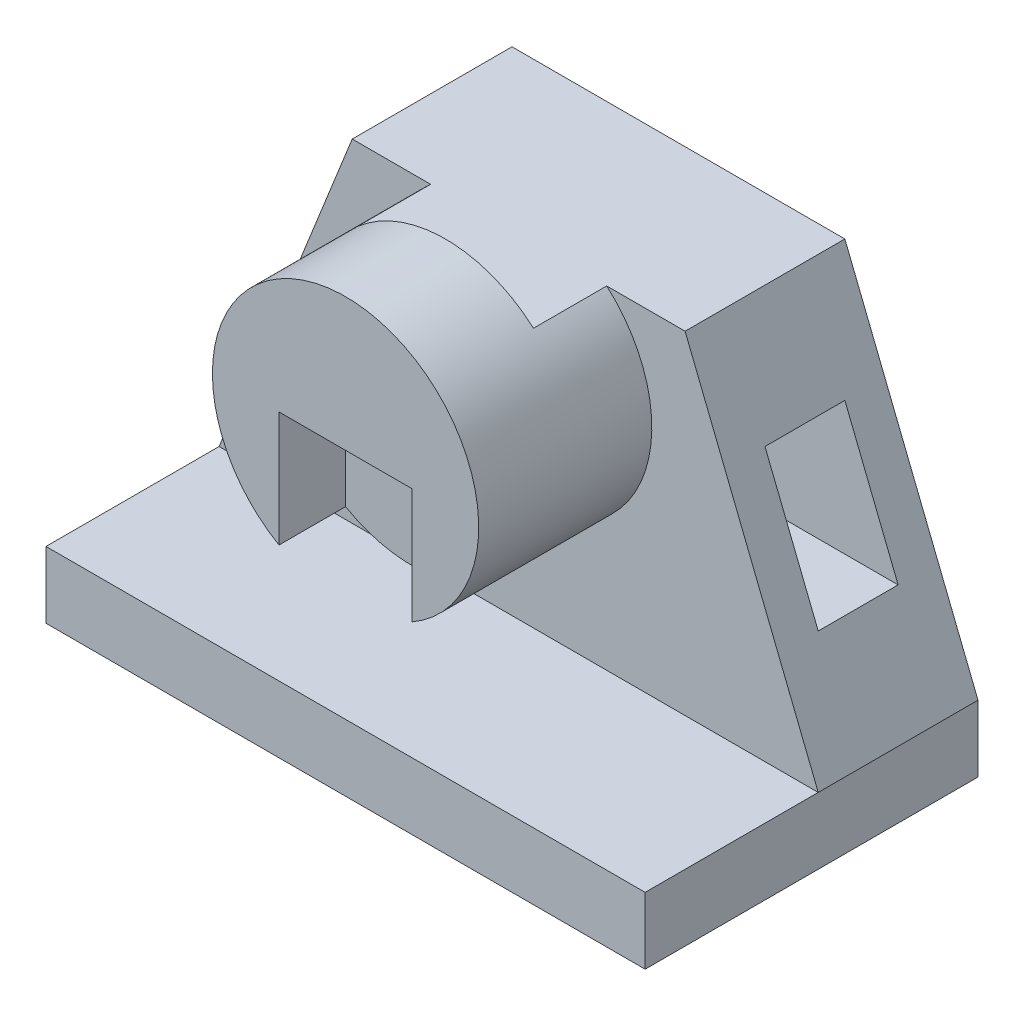
ISO-10303-21;
HEADER;
FILE_DESCRIPTION(('STEP AP214'),'2;1');
FILE_NAME('part.step','',(''),(''),'','','');
FILE_SCHEMA(('AUTOMOTIVE_DESIGN { 1 0 10303 214 1 1 1 1 }'));
ENDSEC;
DATA;
#1=APPLICATION_CONTEXT('core data for automotive mechanical design processes');
#2=APPLICATION_PROTOCOL_DEFINITION('international standard','automotive_design',2000,#1);
#3=PRODUCT_CONTEXT('',#1,'mechanical');
#4=PRODUCT('Part','Part','',(#3));
#5=PRODUCT_RELATED_PRODUCT_CATEGORY('part','',(#4));
#6=PRODUCT_DEFINITION_FORMATION('','',#4);
#7=PRODUCT_DEFINITION_CONTEXT('part definition',#1,'design');
#8=PRODUCT_DEFINITION('design','',#6,#7);
#9=PRODUCT_DEFINITION_SHAPE('','',#8);
#10=(LENGTH_UNIT() NAMED_UNIT(*) SI_UNIT(.MILLI.,.METRE.));
#11=(NAMED_UNIT(*) PLANE_ANGLE_UNIT() SI_UNIT($,.RADIAN.));
#12=(NAMED_UNIT(*) SI_UNIT($,.STERADIAN.) SOLID_ANGLE_UNIT());
#13=UNCERTAINTY_MEASURE_WITH_UNIT(LENGTH_MEASURE(1.E-05),#10,'distance_accuracy_value','');
#14=(GEOMETRIC_REPRESENTATION_CONTEXT(3) GLOBAL_UNCERTAINTY_ASSIGNED_CONTEXT((#13)) GLOBAL_UNIT_ASSIGNED_CONTEXT((#10,
#11,#12)) REPRESENTATION_CONTEXT('',''));
#15=CARTESIAN_POINT('',(0.,0.,0.));
#16=DIRECTION('',(0.,0.,1.));
#17=DIRECTION('',(1.,0.,0.));
#18=AXIS2_PLACEMENT_3D('',#15,#16,#17);
#19=CARTESIAN_POINT('',(-3.44827586206896,1.37931034482759,24.));
#20=DIRECTION('',(-0.928476690885259,0.371390676354103,0.));
#21=DIRECTION('',(-0.371390676354104,-0.928476690885259,0.));
#22=AXIS2_PLACEMENT_3D('',#19,#20,#21);
#23=PLANE('',#22);
#24=DIRECTION('',(0.371390676354104,0.92847669088526,0.));
#25=VECTOR('',#24,1.);
#26=CARTESIAN_POINT('',(-3.44827586206896,1.37931034482759,18.));
#27=LINE('',#26,#25);
#28=CARTESIAN_POINT('',(5.99999999999999,25.,18.));
#29=VERTEX_POINT('',#28);
#30=CARTESIAN_POINT('',(14.,45.,18.));
#31=VERTEX_POINT('',#30);
#32=EDGE_CURVE('E167',#29,#31,#27,.T.);
#33=ORIENTED_EDGE('',*,*,#32,.F.);
#34=DIRECTION('',(0.,0.,1.));
#35=VECTOR('',#34,1.);
#36=CARTESIAN_POINT('',(5.99999999999999,25.,24.));
#37=LINE('',#36,#35);
#38=CARTESIAN_POINT('',(5.99999999999999,25.,6.00000000000001));
#39=VERTEX_POINT('',#38);
#40=EDGE_CURVE('E154',#39,#29,#37,.T.);
#41=ORIENTED_EDGE('',*,*,#40,.F.);
#42=DIRECTION('',(-0.371390676354104,-0.92847669088526,0.));
#43=VECTOR('',#42,1.);
#44=CARTESIAN_POINT('',(-3.44827586206896,1.37931034482759,6.));
#45=LINE('',#44,#43);
#46=CARTESIAN_POINT('',(14.,45.,6.00000000000001));
#47=VERTEX_POINT('',#46);
#48=EDGE_CURVE('E159',#47,#39,#45,.T.);
#49=ORIENTED_EDGE('',*,*,#48,.F.);
#50=DIRECTION('',(0.,0.,-1.));
#51=VECTOR('',#50,1.);
#52=CARTESIAN_POINT('',(14.,45.,24.));
#53=LINE('',#52,#51);
#54=EDGE_CURVE('E171',#31,#47,#53,.T.);
#55=ORIENTED_EDGE('',*,*,#54,.F.);
#56=EDGE_LOOP('',(#33,#41,#49,#55));
#57=FACE_BOUND('',#56,.T.);
#58=DIRECTION('',(0.371390676354104,0.928476690885259,0.));
#59=VECTOR('',#58,1.);
#60=CARTESIAN_POINT('',(-3.44827586206896,1.37931034482759,0.));
#61=LINE('',#60,#59);
#62=CARTESIAN_POINT('',(0.,10.,0.));
#63=VERTEX_POINT('',#62);
#64=CARTESIAN_POINT('',(20.,60.,0.));
#65=VERTEX_POINT('',#64);
#66=EDGE_CURVE('E242',#63,#65,#61,.T.);
#67=ORIENTED_EDGE('',*,*,#66,.F.);
#68=DIRECTION('',(0.,0.,-1.));
#69=VECTOR('',#68,1.);
#70=CARTESIAN_POINT('',(0.,10.,24.));
#71=LINE('',#70,#69);
#72=CARTESIAN_POINT('',(0.,10.,24.));
#73=VERTEX_POINT('',#72);
#74=EDGE_CURVE('E273',#73,#63,#71,.T.);
#75=ORIENTED_EDGE('',*,*,#74,.F.);
#76=DIRECTION('',(0.371390676354104,0.928476690885259,0.));
#77=VECTOR('',#76,1.);
#78=CARTESIAN_POINT('',(-3.44827586206896,1.37931034482759,24.));
#79=LINE('',#78,#77);
#80=CARTESIAN_POINT('',(20.,60.,24.));
#81=VERTEX_POINT('',#80);
#82=EDGE_CURVE('E247',#73,#81,#79,.T.);
#83=ORIENTED_EDGE('',*,*,#82,.T.);
#84=DIRECTION('',(0.,0.,-1.));
#85=VECTOR('',#84,1.);
#86=CARTESIAN_POINT('',(20.,60.,24.));
#87=LINE('',#86,#85);
#88=EDGE_CURVE('E257',#81,#65,#87,.T.);
#89=ORIENTED_EDGE('',*,*,#88,.T.);
#90=EDGE_LOOP('',(#67,#75,#83,#89));
#91=FACE_BOUND('',#90,.T.);
#92=ADVANCED_FACE('F41',(#57,#91),#23,.T.);
#93=CARTESIAN_POINT('',(81.0344827586207,32.4137931034483,24.));
#94=DIRECTION('',(0.928476690885259,0.371390676354104,0.));
#95=DIRECTION('',(-0.371390676354104,0.928476690885259,0.));
#96=AXIS2_PLACEMENT_3D('',#93,#94,#95);
#97=PLANE('',#96);
#98=DIRECTION('',(0.371390676354104,-0.928476690885259,0.));
#99=VECTOR('',#98,1.);
#100=CARTESIAN_POINT('',(81.0344827586207,32.4137931034483,18.));
#101=LINE('',#100,#99);
#102=CARTESIAN_POINT('',(76.,45.,18.));
#103=VERTEX_POINT('',#102);
#104=CARTESIAN_POINT('',(84.,25.,18.));
#105=VERTEX_POINT('',#104);
#106=EDGE_CURVE('E11',#103,#105,#101,.T.);
#107=ORIENTED_EDGE('',*,*,#106,.F.);
#108=DIRECTION('',(0.,0.,1.));
#109=VECTOR('',#108,1.);
#110=CARTESIAN_POINT('',(76.,45.,24.));
#111=LINE('',#110,#109);
#112=CARTESIAN_POINT('',(76.,45.,6.00000000000001));
#113=VERTEX_POINT('',#112);
#114=EDGE_CURVE('E48',#113,#103,#111,.T.);
#115=ORIENTED_EDGE('',*,*,#114,.F.);
#116=DIRECTION('',(-0.371390676354104,0.928476690885259,0.));
#117=VECTOR('',#116,1.);
#118=CARTESIAN_POINT('',(81.0344827586207,32.4137931034483,6.00000000000001));
#119=LINE('',#118,#117);
#120=CARTESIAN_POINT('',(84.,25.,6.));
#121=VERTEX_POINT('',#120);
#122=EDGE_CURVE('E283',#121,#113,#119,.T.);
#123=ORIENTED_EDGE('',*,*,#122,.F.);
#124=DIRECTION('',(0.,0.,-1.));
#125=VECTOR('',#124,1.);
#126=CARTESIAN_POINT('',(84.,25.,24.));
#127=LINE('',#126,#125);
#128=EDGE_CURVE('E276',#105,#121,#127,.T.);
#129=ORIENTED_EDGE('',*,*,#128,.F.);
#130=EDGE_LOOP('',(#107,#115,#123,#129));
#131=FACE_BOUND('',#130,.T.);
#132=DIRECTION('',(0.371390676354104,-0.928476690885259,0.));
#133=VECTOR('',#132,1.);
#134=CARTESIAN_POINT('',(81.0344827586207,32.4137931034483,0.));
#135=LINE('',#134,#133);
#136=CARTESIAN_POINT('',(70.,60.,0.));
#137=VERTEX_POINT('',#136);
#138=CARTESIAN_POINT('',(90.,10.,0.));
#139=VERTEX_POINT('',#138);
#140=EDGE_CURVE('E263',#137,#139,#135,.T.);
#141=ORIENTED_EDGE('',*,*,#140,.F.);
#142=DIRECTION('',(0.,0.,-1.));
#143=VECTOR('',#142,1.);
#144=CARTESIAN_POINT('',(70.,60.,24.));
#145=LINE('',#144,#143);
#146=CARTESIAN_POINT('',(70.,60.,24.));
#147=VERTEX_POINT('',#146);
#148=EDGE_CURVE('E267',#147,#137,#145,.T.);
#149=ORIENTED_EDGE('',*,*,#148,.F.);
#150=DIRECTION('',(0.371390676354104,-0.928476690885259,0.));
#151=VECTOR('',#150,1.);
#152=CARTESIAN_POINT('',(81.0344827586207,32.4137931034483,24.));
#153=LINE('',#152,#151);
#154=CARTESIAN_POINT('',(90.,10.,24.));
#155=VERTEX_POINT('',#154);
#156=EDGE_CURVE('E251',#147,#155,#153,.T.);
#157=ORIENTED_EDGE('',*,*,#156,.T.);
#158=DIRECTION('',(0.,0.,-1.));
#159=VECTOR('',#158,1.);
#160=CARTESIAN_POINT('',(90.,10.,24.));
#161=LINE('',#160,#159);
#162=EDGE_CURVE('E271',#155,#139,#161,.T.);
#163=ORIENTED_EDGE('',*,*,#162,.T.);
#164=EDGE_LOOP('',(#141,#149,#157,#163));
#165=FACE_BOUND('',#164,.T.);
#166=ADVANCED_FACE('F292',(#131,#165),#97,.T.);
#167=CARTESIAN_POINT('',(0.,60.,24.));
#168=DIRECTION('',(0.,1.,0.));
#169=DIRECTION('',(-1.,0.,0.));
#170=AXIS2_PLACEMENT_3D('',#167,#168,#169);
#171=PLANE('',#170);
#172=DIRECTION('',(1.,0.,0.));
#173=VECTOR('',#172,1.);
#174=CARTESIAN_POINT('',(0.,60.,0.));
#175=LINE('',#174,#173);
#176=EDGE_CURVE('E248',#65,#137,#175,.T.);
#177=ORIENTED_EDGE('',*,*,#176,.F.);
#178=ORIENTED_EDGE('',*,*,#88,.F.);
#179=DIRECTION('',(1.,0.,0.));
#180=VECTOR('',#179,1.);
#181=CARTESIAN_POINT('',(0.,60.,24.));
#182=LINE('',#181,#180);
#183=CARTESIAN_POINT('',(31.7712434446771,60.,24.));
#184=VERTEX_POINT('',#183);
#185=EDGE_CURVE('E260',#81,#184,#182,.T.);
#186=ORIENTED_EDGE('',*,*,#185,.T.);
#187=DIRECTION('',(0.,0.,-1.));
#188=VECTOR('',#187,1.);
#189=CARTESIAN_POINT('',(31.7712434446771,60.,35.));
#190=LINE('',#189,#188);
#191=CARTESIAN_POINT('',(31.7712434446771,60.,35.));
#192=VERTEX_POINT('',#191);
#193=EDGE_CURVE('E184',#192,#184,#190,.T.);
#194=ORIENTED_EDGE('',*,*,#193,.F.);
#195=DIRECTION('',(-1.,0.,0.));
#196=VECTOR('',#195,1.);
#197=CARTESIAN_POINT('',(58.2287565553229,60.,35.));
#198=LINE('',#197,#196);
#199=CARTESIAN_POINT('',(58.2287565553229,60.,35.));
#200=VERTEX_POINT('',#199);
#201=EDGE_CURVE('E177',#200,#192,#198,.T.);
#202=ORIENTED_EDGE('',*,*,#201,.F.);
#203=DIRECTION('',(0.,0.,-1.));
#204=VECTOR('',#203,1.);
#205=CARTESIAN_POINT('',(58.2287565553229,60.,35.));
#206=LINE('',#205,#204);
#207=CARTESIAN_POINT('',(58.2287565553229,60.,24.));
#208=VERTEX_POINT('',#207);
#209=EDGE_CURVE('E181',#200,#208,#206,.T.);
#210=ORIENTED_EDGE('',*,*,#209,.T.);
#211=EDGE_CURVE('E258',#208,#147,#182,.T.);
#212=ORIENTED_EDGE('',*,*,#211,.T.);
#213=ORIENTED_EDGE('',*,*,#148,.T.);
#214=EDGE_LOOP('',(#177,#178,#186,#194,#202,#210,#212,#213));
#215=FACE_BOUND('',#214,.T.);
#216=ADVANCED_FACE('F309',(#215),#171,.T.);
#217=CARTESIAN_POINT('',(0.,0.,24.));
#218=DIRECTION('',(0.,0.,1.));
#219=DIRECTION('',(1.,0.,0.));
#220=AXIS2_PLACEMENT_3D('',#217,#218,#219);
#221=PLANE('',#220);
#222=ORIENTED_EDGE('',*,*,#211,.F.);
#223=CARTESIAN_POINT('',(45.,45.,24.));
#224=DIRECTION('',(0.,0.,1.));
#225=DIRECTION('',(1.,0.,0.));
#226=AXIS2_PLACEMENT_3D('',#223,#224,#225);
#227=CIRCLE('',#226,20.);
#228=EDGE_CURVE('E277',#208,#184,#227,.F.);
#229=ORIENTED_EDGE('',*,*,#228,.T.);
#230=ORIENTED_EDGE('',*,*,#185,.F.);
#231=ORIENTED_EDGE('',*,*,#82,.F.);
#232=DIRECTION('',(1.,0.,0.));
#233=VECTOR('',#232,1.);
#234=CARTESIAN_POINT('',(0.,10.,24.));
#235=LINE('',#234,#233);
#236=EDGE_CURVE('E246',#73,#155,#235,.T.);
#237=ORIENTED_EDGE('',*,*,#236,.T.);
#238=ORIENTED_EDGE('',*,*,#156,.F.);
#239=EDGE_LOOP('',(#222,#229,#230,#231,#237,#238));
#240=FACE_BOUND('',#239,.T.);
#241=ADVANCED_FACE('F312',(#240),#221,.T.);
#242=CARTESIAN_POINT('',(0.,0.,0.));
#243=DIRECTION('',(0.,0.,1.));
#244=DIRECTION('',(1.,0.,0.));
#245=AXIS2_PLACEMENT_3D('',#242,#243,#244);
#246=PLANE('',#245);
#247=ORIENTED_EDGE('',*,*,#66,.T.);
#248=ORIENTED_EDGE('',*,*,#176,.T.);
#249=ORIENTED_EDGE('',*,*,#140,.T.);
#250=DIRECTION('',(0.,1.,0.));
#251=VECTOR('',#250,1.);
#252=CARTESIAN_POINT('',(90.,0.,0.));
#253=LINE('',#252,#251);
#254=CARTESIAN_POINT('',(90.,0.,0.));
#255=VERTEX_POINT('',#254);
#256=EDGE_CURVE('E221',#255,#139,#253,.T.);
#257=ORIENTED_EDGE('',*,*,#256,.F.);
#258=DIRECTION('',(1.,0.,0.));
#259=VECTOR('',#258,1.);
#260=CARTESIAN_POINT('',(0.,0.,0.));
#261=LINE('',#260,#259);
#262=CARTESIAN_POINT('',(0.,0.,0.));
#263=VERTEX_POINT('',#262);
#264=EDGE_CURVE('E235',#263,#255,#261,.T.);
#265=ORIENTED_EDGE('',*,*,#264,.F.);
#266=DIRECTION('',(0.,-1.,0.));
#267=VECTOR('',#266,1.);
#268=CARTESIAN_POINT('',(0.,10.,0.));
#269=LINE('',#268,#267);
#270=EDGE_CURVE('E218',#63,#263,#269,.T.);
#271=ORIENTED_EDGE('',*,*,#270,.F.);
#272=EDGE_LOOP('',(#247,#248,#249,#257,#265,#271));
#273=FACE_BOUND('',#272,.T.);
#274=ADVANCED_FACE('F317',(#273),#246,.F.);
#275=CARTESIAN_POINT('',(90.,10.,50.));
#276=DIRECTION('',(0.,-1.,0.));
#277=DIRECTION('',(1.,0.,0.));
#278=AXIS2_PLACEMENT_3D('',#275,#276,#277);
#279=PLANE('',#278);
#280=ORIENTED_EDGE('',*,*,#236,.F.);
#281=DIRECTION('',(0.,0.,-1.));
#282=VECTOR('',#281,1.);
#283=CARTESIAN_POINT('',(0.,10.,50.));
#284=LINE('',#283,#282);
#285=CARTESIAN_POINT('',(0.,10.,50.));
#286=VERTEX_POINT('',#285);
#287=EDGE_CURVE('E245',#286,#73,#284,.T.);
#288=ORIENTED_EDGE('',*,*,#287,.F.);
#289=DIRECTION('',(-1.,0.,0.));
#290=VECTOR('',#289,1.);
#291=CARTESIAN_POINT('',(90.,10.,50.));
#292=LINE('',#291,#290);
#293=CARTESIAN_POINT('',(90.,10.,50.));
#294=VERTEX_POINT('',#293);
#295=EDGE_CURVE('E219',#294,#286,#292,.T.);
#296=ORIENTED_EDGE('',*,*,#295,.F.);
#297=DIRECTION('',(0.,0.,-1.));
#298=VECTOR('',#297,1.);
#299=CARTESIAN_POINT('',(90.,10.,50.));
#300=LINE('',#299,#298);
#301=EDGE_CURVE('E227',#294,#155,#300,.T.);
#302=ORIENTED_EDGE('',*,*,#301,.T.);
#303=EDGE_LOOP('',(#280,#288,#296,#302));
#304=FACE_BOUND('',#303,.T.);
#305=ADVANCED_FACE('F325',(#304),#279,.F.);
#306=CARTESIAN_POINT('',(0.,10.,50.));
#307=DIRECTION('',(1.,0.,0.));
#308=DIRECTION('',(0.,0.,-1.));
#309=AXIS2_PLACEMENT_3D('',#306,#307,#308);
#310=PLANE('',#309);
#311=ORIENTED_EDGE('',*,*,#270,.T.);
#312=DIRECTION('',(0.,0.,-1.));
#313=VECTOR('',#312,1.);
#314=CARTESIAN_POINT('',(0.,0.,50.));
#315=LINE('',#314,#313);
#316=CARTESIAN_POINT('',(0.,0.,50.));
#317=VERTEX_POINT('',#316);
#318=EDGE_CURVE('E239',#317,#263,#315,.T.);
#319=ORIENTED_EDGE('',*,*,#318,.F.);
#320=DIRECTION('',(0.,-1.,0.));
#321=VECTOR('',#320,1.);
#322=CARTESIAN_POINT('',(0.,10.,50.));
#323=LINE('',#322,#321);
#324=EDGE_CURVE('E224',#286,#317,#323,.T.);
#325=ORIENTED_EDGE('',*,*,#324,.F.);
#326=ORIENTED_EDGE('',*,*,#287,.T.);
#327=ORIENTED_EDGE('',*,*,#74,.T.);
#328=EDGE_LOOP('',(#311,#319,#325,#326,#327));
#329=FACE_BOUND('',#328,.T.);
#330=ADVANCED_FACE('F328',(#329),#310,.F.);
#331=CARTESIAN_POINT('',(0.,0.,50.));
#332=DIRECTION('',(0.,1.,0.));
#333=DIRECTION('',(0.,0.,1.));
#334=AXIS2_PLACEMENT_3D('',#331,#332,#333);
#335=PLANE('',#334);
#336=ORIENTED_EDGE('',*,*,#264,.T.);
#337=DIRECTION('',(0.,0.,-1.));
#338=VECTOR('',#337,1.);
#339=CARTESIAN_POINT('',(90.,0.,50.));
#340=LINE('',#339,#338);
#341=CARTESIAN_POINT('',(90.,0.,50.));
#342=VERTEX_POINT('',#341);
#343=EDGE_CURVE('E237',#342,#255,#340,.T.);
#344=ORIENTED_EDGE('',*,*,#343,.F.);
#345=DIRECTION('',(1.,0.,0.));
#346=VECTOR('',#345,1.);
#347=CARTESIAN_POINT('',(0.,0.,50.));
#348=LINE('',#347,#346);
#349=EDGE_CURVE('E228',#317,#342,#348,.T.);
#350=ORIENTED_EDGE('',*,*,#349,.F.);
#351=ORIENTED_EDGE('',*,*,#318,.T.);
#352=EDGE_LOOP('',(#336,#344,#350,#351));
#353=FACE_BOUND('',#352,.T.);
#354=ADVANCED_FACE('F334',(#353),#335,.F.);
#355=CARTESIAN_POINT('',(90.,0.,50.));
#356=DIRECTION('',(-1.,0.,0.));
#357=DIRECTION('',(0.,0.,1.));
#358=AXIS2_PLACEMENT_3D('',#355,#356,#357);
#359=PLANE('',#358);
#360=ORIENTED_EDGE('',*,*,#256,.T.);
#361=ORIENTED_EDGE('',*,*,#162,.F.);
#362=ORIENTED_EDGE('',*,*,#301,.F.);
#363=DIRECTION('',(0.,1.,0.));
#364=VECTOR('',#363,1.);
#365=CARTESIAN_POINT('',(90.,0.,50.));
#366=LINE('',#365,#364);
#367=EDGE_CURVE('E226',#342,#294,#366,.T.);
#368=ORIENTED_EDGE('',*,*,#367,.F.);
#369=ORIENTED_EDGE('',*,*,#343,.T.);
#370=EDGE_LOOP('',(#360,#361,#362,#368,#369));
#371=FACE_BOUND('',#370,.T.);
#372=ADVANCED_FACE('F340',(#371),#359,.F.);
#373=CARTESIAN_POINT('',(0.,0.,50.));
#374=DIRECTION('',(0.,0.,1.));
#375=DIRECTION('',(1.,0.,0.));
#376=AXIS2_PLACEMENT_3D('',#373,#374,#375);
#377=PLANE('',#376);
#378=ORIENTED_EDGE('',*,*,#295,.T.);
#379=ORIENTED_EDGE('',*,*,#324,.T.);
#380=ORIENTED_EDGE('',*,*,#349,.T.);
#381=ORIENTED_EDGE('',*,*,#367,.T.);
#382=EDGE_LOOP('',(#378,#379,#380,#381));
#383=FACE_BOUND('',#382,.T.);
#384=ADVANCED_FACE('F342',(#383),#377,.T.);
#385=CARTESIAN_POINT('',(45.,45.,50.));
#386=DIRECTION('',(0.,0.,-1.));
#387=DIRECTION('',(-1.,0.,0.));
#388=AXIS2_PLACEMENT_3D('',#385,#386,#387);
#389=CYLINDRICAL_SURFACE('',#388,20.);
#390=CARTESIAN_POINT('',(45.,45.,50.));
#391=DIRECTION('',(0.,0.,1.));
#392=DIRECTION('',(1.,0.,0.));
#393=AXIS2_PLACEMENT_3D('',#390,#391,#392);
#394=CIRCLE('',#393,20.);
#395=CARTESIAN_POINT('',(55.,27.6794919243112,50.));
#396=VERTEX_POINT('',#395);
#397=CARTESIAN_POINT('',(35.,27.6794919243112,50.));
#398=VERTEX_POINT('',#397);
#399=EDGE_CURVE('E207',#396,#398,#394,.T.);
#400=ORIENTED_EDGE('',*,*,#399,.F.);
#401=DIRECTION('',(0.,0.,1.));
#402=VECTOR('',#401,1.);
#403=CARTESIAN_POINT('',(55.,27.6794919243112,40.));
#404=LINE('',#403,#402);
#405=CARTESIAN_POINT('',(55.,27.6794919243112,40.));
#406=VERTEX_POINT('',#405);
#407=EDGE_CURVE('E210',#406,#396,#404,.T.);
#408=ORIENTED_EDGE('',*,*,#407,.F.);
#409=CARTESIAN_POINT('',(45.,45.,40.));
#410=DIRECTION('',(0.,0.,1.));
#411=DIRECTION('',(1.,0.,0.));
#412=AXIS2_PLACEMENT_3D('',#409,#410,#411);
#413=CIRCLE('',#412,20.);
#414=CARTESIAN_POINT('',(35.,27.6794919243112,40.));
#415=VERTEX_POINT('',#414);
#416=EDGE_CURVE('E196',#415,#406,#413,.T.);
#417=ORIENTED_EDGE('',*,*,#416,.F.);
#418=DIRECTION('',(0.,0.,1.));
#419=VECTOR('',#418,1.);
#420=CARTESIAN_POINT('',(35.,27.6794919243112,40.));
#421=LINE('',#420,#419);
#422=EDGE_CURVE('E209',#415,#398,#421,.T.);
#423=ORIENTED_EDGE('',*,*,#422,.T.);
#424=EDGE_LOOP('',(#400,#408,#417,#423));
#425=FACE_BOUND('',#424,.T.);
#426=CARTESIAN_POINT('',(45.,45.,35.));
#427=DIRECTION('',(0.,0.,-1.));
#428=DIRECTION('',(-1.,0.,0.));
#429=AXIS2_PLACEMENT_3D('',#426,#427,#428);
#430=CIRCLE('',#429,20.);
#431=EDGE_CURVE('E174',#192,#200,#430,.T.);
#432=ORIENTED_EDGE('',*,*,#431,.F.);
#433=ORIENTED_EDGE('',*,*,#193,.T.);
#434=ORIENTED_EDGE('',*,*,#228,.F.);
#435=ORIENTED_EDGE('',*,*,#209,.F.);
#436=EDGE_LOOP('',(#432,#433,#434,#435));
#437=FACE_BOUND('',#436,.T.);
#438=ADVANCED_FACE('F343',(#425,#437),#389,.T.);
#439=CARTESIAN_POINT('',(45.,45.,50.));
#440=DIRECTION('',(0.,0.,1.));
#441=DIRECTION('',(1.,0.,0.));
#442=AXIS2_PLACEMENT_3D('',#439,#440,#441);
#443=PLANE('',#442);
#444=DIRECTION('',(0.,1.,0.));
#445=VECTOR('',#444,1.);
#446=CARTESIAN_POINT('',(55.,45.,50.));
#447=LINE('',#446,#445);
#448=CARTESIAN_POINT('',(55.,45.,50.));
#449=VERTEX_POINT('',#448);
#450=EDGE_CURVE('E188',#396,#449,#447,.T.);
#451=ORIENTED_EDGE('',*,*,#450,.F.);
#452=ORIENTED_EDGE('',*,*,#399,.T.);
#453=DIRECTION('',(0.,-1.,0.));
#454=VECTOR('',#453,1.);
#455=CARTESIAN_POINT('',(35.,45.,50.));
#456=LINE('',#455,#454);
#457=CARTESIAN_POINT('',(35.,45.,50.));
#458=VERTEX_POINT('',#457);
#459=EDGE_CURVE('E195',#458,#398,#456,.T.);
#460=ORIENTED_EDGE('',*,*,#459,.F.);
#461=DIRECTION('',(-1.,0.,0.));
#462=VECTOR('',#461,1.);
#463=CARTESIAN_POINT('',(35.,45.,50.));
#464=LINE('',#463,#462);
#465=EDGE_CURVE('E201',#449,#458,#464,.T.);
#466=ORIENTED_EDGE('',*,*,#465,.F.);
#467=EDGE_LOOP('',(#451,#452,#460,#466));
#468=FACE_BOUND('',#467,.T.);
#469=ADVANCED_FACE('F349',(#468),#443,.T.);
#470=CARTESIAN_POINT('',(55.,45.,40.));
#471=DIRECTION('',(1.,0.,0.));
#472=DIRECTION('',(0.,1.,0.));
#473=AXIS2_PLACEMENT_3D('',#470,#471,#472);
#474=PLANE('',#473);
#475=ORIENTED_EDGE('',*,*,#450,.T.);
#476=DIRECTION('',(0.,0.,1.));
#477=VECTOR('',#476,1.);
#478=CARTESIAN_POINT('',(55.,45.,40.));
#479=LINE('',#478,#477);
#480=CARTESIAN_POINT('',(55.,45.,40.));
#481=VERTEX_POINT('',#480);
#482=EDGE_CURVE('E203',#481,#449,#479,.T.);
#483=ORIENTED_EDGE('',*,*,#482,.F.);
#484=DIRECTION('',(0.,1.,0.));
#485=VECTOR('',#484,1.);
#486=CARTESIAN_POINT('',(55.,45.,40.));
#487=LINE('',#486,#485);
#488=EDGE_CURVE('E186',#406,#481,#487,.T.);
#489=ORIENTED_EDGE('',*,*,#488,.F.);
#490=ORIENTED_EDGE('',*,*,#407,.T.);
#491=EDGE_LOOP('',(#475,#483,#489,#490));
#492=FACE_BOUND('',#491,.T.);
#493=ADVANCED_FACE('F351',(#492),#474,.F.);
#494=CARTESIAN_POINT('',(35.,45.,40.));
#495=DIRECTION('',(-1.,0.,0.));
#496=DIRECTION('',(0.,-1.,0.));
#497=AXIS2_PLACEMENT_3D('',#494,#495,#496);
#498=PLANE('',#497);
#499=ORIENTED_EDGE('',*,*,#459,.T.);
#500=ORIENTED_EDGE('',*,*,#422,.F.);
#501=DIRECTION('',(0.,-1.,0.));
#502=VECTOR('',#501,1.);
#503=CARTESIAN_POINT('',(35.,45.,40.));
#504=LINE('',#503,#502);
#505=CARTESIAN_POINT('',(35.,45.,40.));
#506=VERTEX_POINT('',#505);
#507=EDGE_CURVE('E193',#506,#415,#504,.T.);
#508=ORIENTED_EDGE('',*,*,#507,.F.);
#509=DIRECTION('',(0.,0.,1.));
#510=VECTOR('',#509,1.);
#511=CARTESIAN_POINT('',(35.,45.,40.));
#512=LINE('',#511,#510);
#513=EDGE_CURVE('E213',#506,#458,#512,.T.);
#514=ORIENTED_EDGE('',*,*,#513,.T.);
#515=EDGE_LOOP('',(#499,#500,#508,#514));
#516=FACE_BOUND('',#515,.T.);
#517=ADVANCED_FACE('F360',(#516),#498,.F.);
#518=CARTESIAN_POINT('',(35.,45.,40.));
#519=DIRECTION('',(0.,1.,0.));
#520=DIRECTION('',(0.,0.,1.));
#521=AXIS2_PLACEMENT_3D('',#518,#519,#520);
#522=PLANE('',#521);
#523=ORIENTED_EDGE('',*,*,#465,.T.);
#524=ORIENTED_EDGE('',*,*,#513,.F.);
#525=DIRECTION('',(-1.,0.,0.));
#526=VECTOR('',#525,1.);
#527=CARTESIAN_POINT('',(35.,45.,40.));
#528=LINE('',#527,#526);
#529=EDGE_CURVE('E192',#481,#506,#528,.T.);
#530=ORIENTED_EDGE('',*,*,#529,.F.);
#531=ORIENTED_EDGE('',*,*,#482,.T.);
#532=EDGE_LOOP('',(#523,#524,#530,#531));
#533=FACE_BOUND('',#532,.T.);
#534=ADVANCED_FACE('F356',(#533),#522,.F.);
#535=CARTESIAN_POINT('',(45.,45.,40.));
#536=DIRECTION('',(0.,0.,1.));
#537=DIRECTION('',(1.,0.,0.));
#538=AXIS2_PLACEMENT_3D('',#535,#536,#537);
#539=PLANE('',#538);
#540=ORIENTED_EDGE('',*,*,#488,.T.);
#541=ORIENTED_EDGE('',*,*,#529,.T.);
#542=ORIENTED_EDGE('',*,*,#507,.T.);
#543=ORIENTED_EDGE('',*,*,#416,.T.);
#544=EDGE_LOOP('',(#540,#541,#542,#543));
#545=FACE_BOUND('',#544,.T.);
#546=ADVANCED_FACE('F362',(#545),#539,.T.);
#547=CARTESIAN_POINT('',(45.,45.,35.));
#548=DIRECTION('',(0.,0.,-1.));
#549=DIRECTION('',(-1.,0.,0.));
#550=AXIS2_PLACEMENT_3D('',#547,#548,#549);
#551=PLANE('',#550);
#552=ORIENTED_EDGE('',*,*,#431,.T.);
#553=ORIENTED_EDGE('',*,*,#201,.T.);
#554=EDGE_LOOP('',(#552,#553));
#555=FACE_BOUND('',#554,.T.);
#556=ADVANCED_FACE('F369',(#555),#551,.T.);
#557=CARTESIAN_POINT('',(0.,45.,18.));
#558=DIRECTION('',(0.,0.,1.));
#559=DIRECTION('',(0.,-1.,0.));
#560=AXIS2_PLACEMENT_3D('',#557,#558,#559);
#561=PLANE('',#560);
#562=ORIENTED_EDGE('',*,*,#32,.T.);
#563=DIRECTION('',(1.,0.,0.));
#564=VECTOR('',#563,1.);
#565=CARTESIAN_POINT('',(0.,45.,18.));
#566=LINE('',#565,#564);
#567=EDGE_CURVE('E161',#31,#103,#566,.T.);
#568=ORIENTED_EDGE('',*,*,#567,.T.);
#569=ORIENTED_EDGE('',*,*,#106,.T.);
#570=DIRECTION('',(1.,0.,0.));
#571=VECTOR('',#570,1.);
#572=CARTESIAN_POINT('',(0.,25.,18.));
#573=LINE('',#572,#571);
#574=EDGE_CURVE('E58',#29,#105,#573,.T.);
#575=ORIENTED_EDGE('',*,*,#574,.F.);
#576=EDGE_LOOP('',(#562,#568,#569,#575));
#577=FACE_BOUND('',#576,.T.);
#578=ADVANCED_FACE('F163',(#577),#561,.F.);
#579=CARTESIAN_POINT('',(0.,45.,18.));
#580=DIRECTION('',(0.,1.,0.));
#581=DIRECTION('',(0.,0.,1.));
#582=AXIS2_PLACEMENT_3D('',#579,#580,#581);
#583=PLANE('',#582);
#584=ORIENTED_EDGE('',*,*,#54,.T.);
#585=DIRECTION('',(1.,0.,0.));
#586=VECTOR('',#585,1.);
#587=CARTESIAN_POINT('',(0.,45.,6.00000000000001));
#588=LINE('',#587,#586);
#589=EDGE_CURVE('E290',#47,#113,#588,.T.);
#590=ORIENTED_EDGE('',*,*,#589,.T.);
#591=ORIENTED_EDGE('',*,*,#114,.T.);
#592=ORIENTED_EDGE('',*,*,#567,.F.);
#593=EDGE_LOOP('',(#584,#590,#591,#592));
#594=FACE_BOUND('',#593,.T.);
#595=ADVANCED_FACE('F282',(#594),#583,.F.);
#596=CARTESIAN_POINT('',(0.,45.,6.00000000000001));
#597=DIRECTION('',(0.,0.,-1.));
#598=DIRECTION('',(0.,1.,0.));
#599=AXIS2_PLACEMENT_3D('',#596,#597,#598);
#600=PLANE('',#599);
#601=ORIENTED_EDGE('',*,*,#48,.T.);
#602=DIRECTION('',(1.,0.,0.));
#603=VECTOR('',#602,1.);
#604=CARTESIAN_POINT('',(0.,25.,6.));
#605=LINE('',#604,#603);
#606=EDGE_CURVE('E54',#39,#121,#605,.T.);
#607=ORIENTED_EDGE('',*,*,#606,.T.);
#608=ORIENTED_EDGE('',*,*,#122,.T.);
#609=ORIENTED_EDGE('',*,*,#589,.F.);
#610=EDGE_LOOP('',(#601,#607,#608,#609));
#611=FACE_BOUND('',#610,.T.);
#612=ADVANCED_FACE('F294',(#611),#600,.F.);
#613=CARTESIAN_POINT('',(0.,25.,18.));
#614=DIRECTION('',(0.,-1.,0.));
#615=DIRECTION('',(0.,0.,-1.));
#616=AXIS2_PLACEMENT_3D('',#613,#614,#615);
#617=PLANE('',#616);
#618=ORIENTED_EDGE('',*,*,#40,.T.);
#619=ORIENTED_EDGE('',*,*,#574,.T.);
#620=ORIENTED_EDGE('',*,*,#128,.T.);
#621=ORIENTED_EDGE('',*,*,#606,.F.);
#622=EDGE_LOOP('',(#618,#619,#620,#621));
#623=FACE_BOUND('',#622,.T.);
#624=ADVANCED_FACE('F156',(#623),#617,.F.);
#625=CLOSED_SHELL('',(#92,#166,#216,#241,#274,#305,#330,#354,#372,#384,#438,#469,#493,#517,#534,
#546,#556,#578,#595,#612,#624));
#626=MANIFOLD_SOLID_BREP('B2',#625);
#627=ADVANCED_BREP_SHAPE_REPRESENTATION('',(#18,#626),#14);
#628=SHAPE_DEFINITION_REPRESENTATION(#9,#627);
ENDSEC;
END-ISO-10303-21;
